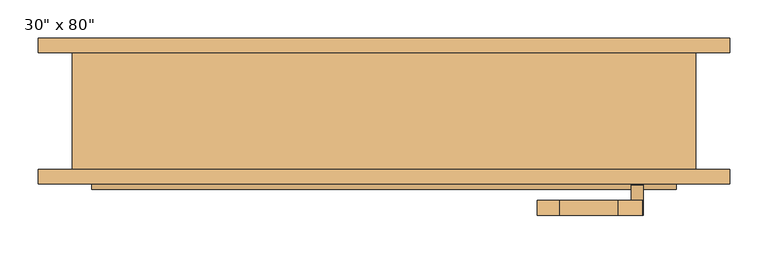
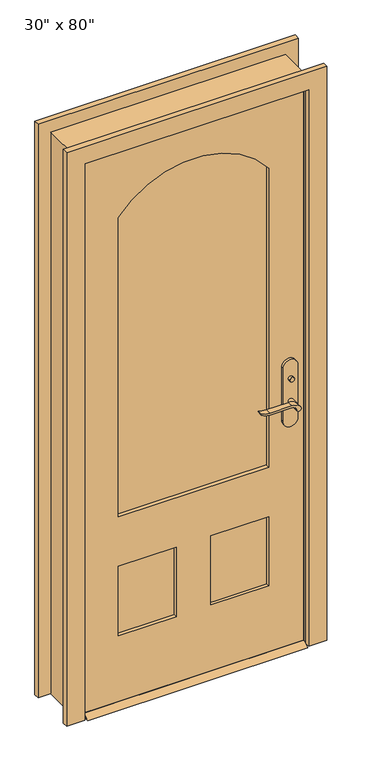
"""IFC4 building model written with IfcOpenShell, lengths in millimetres: door geometry."""

from ifc_helpers import new_model, si_unit, point, frame, frame_2d, origin, place, context, project, spatial, polyline, circle_curve, trimmed, segment, composite_curve, outline, extrude, faceted_brep, source, transform, mapped, element, save


def door_4b146b56(model_context):
    return source(origin(), model_context, "Body", "SolidModel", [
        extrude(outline(polyline([(-38.1, 12.7), (-12.7, 0.0), (-98.425, 0.0), (-73.025, 12.7), (-38.1, 12.7)])), frame((-381.0, 0.0, 0.0), z_axis=(1.0, 0.0, 0.0), x_axis=(0.0, 1.0, 0.0)), (0.0, 0.0, 1.0), 762.0),
        extrude(outline(polyline([(335.2, -18.1), (335.2, -28.1), (325.2, -28.1), (325.2, -18.1), (335.2, -18.1)])), frame((0.0, 0.0, 981.9), z_axis=(0.0, 0.0, 1.0), x_axis=(1.0, 0.0, 0.0)), (0.0, 0.0, 1.0), 30.0),
        extrude(outline(composite_curve([segment(trimmed(circle_curve(frame_2d((996.9, 330.2)), 8.0), [point((996.9, 322.2))], [point((996.9, 338.2))], False, "CARTESIAN"), True, "CONTINUOUS"), segment(trimmed(circle_curve(frame_2d((996.9, 330.2)), 8.0), [point((996.9, 338.2))], [point((996.9, 322.2))], False, "CARTESIAN"), True, "CONTINUOUS")], self_intersect=False)), frame((0.0, -93.025, 0.0), z_axis=(0.0, 1.0, 0.0), x_axis=(0.0, 0.0, 1.0)), (0.0, 0.0, 1.0), 10.0),
        extrude(outline(composite_curve([segment(trimmed(circle_curve(frame_2d((897.1555521, 306.5324871)), 37.2832219), [point((919.0523287, 336.7081363))], [point((934.4, 304.8325667))], False, "CARTESIAN"), True, "CONTINUOUS"), segment(polyline([(934.4, 304.8325667), (934.4, 228.5564091)]), True, "CONTINUOUS"), segment(trimmed(circle_curve(frame_2d((1017.6850638, 228.6227909)), 83.2850902), [point((934.4, 228.5564091))], [point((939.4, 200.2))], True, "CARTESIAN"), True, "CONTINUOUS"), segment(polyline([(939.4, 200.2), (936.6135558, 200.2)]), True, "CONTINUOUS"), segment(trimmed(circle_curve(frame_2d((986.6709207, 232.1396612)), 59.3791355), [point((936.6135558, 200.2))], [point((927.4, 228.5564091))], False, "CARTESIAN"), True, "CONTINUOUS"), segment(polyline([(927.4, 228.5564091), (927.4, 304.8138099)]), True, "CONTINUOUS"), segment(trimmed(circle_curve(frame_2d((909.2738613, 304.8138099)), 18.1261387), [point((927.4, 304.8138099))], [point((914.4, 322.2))], True, "CARTESIAN"), True, "CONTINUOUS"), segment(trimmed(circle_curve(frame_2d((914.4, 330.2)), 8.0), [point((914.4, 322.2))], [point((919.0523287, 336.7081363))], False, "CARTESIAN"), True, "CONTINUOUS")], self_intersect=False)), frame((0.0, 1.9, 0.0), z_axis=(0.0, 1.0, 0.0), x_axis=(0.0, 0.0, 1.0)), (0.0, 0.0, 1.0), 20.0),
        extrude(outline(composite_curve([segment(trimmed(circle_curve(frame_2d((914.4, 330.2)), 8.0), [point((914.3999903, 322.2))], [point((919.0523287, 336.7081363))], False, "CARTESIAN"), True, "CONTINUOUS"), segment(trimmed(circle_curve(frame_2d((897.1555521, 306.5324871)), 37.2832219), [point((919.0523287, 336.7081363))], [point((934.4, 304.8325667))], False, "CARTESIAN"), True, "CONTINUOUS"), segment(polyline([(934.4, 304.8325667), (934.4, 228.5564091)]), True, "CONTINUOUS"), segment(trimmed(circle_curve(frame_2d((1017.6850638, 228.6227909)), 83.2850902), [point((934.4, 228.5564091))], [point((939.4, 200.2))], True, "CARTESIAN"), True, "CONTINUOUS"), segment(polyline([(939.4, 200.2), (936.6135558, 200.2)]), True, "CONTINUOUS"), segment(trimmed(circle_curve(frame_2d((986.6709207, 232.1396612)), 59.3791355), [point((936.6135558, 200.2))], [point((927.4, 228.5564091))], False, "CARTESIAN"), True, "CONTINUOUS"), segment(polyline([(927.4, 228.5564091), (927.4, 304.8138122)]), True, "CONTINUOUS"), segment(trimmed(circle_curve(frame_2d((909.2738682, 304.8138122)), 18.1261318), [point((927.4, 304.8138122))], [point((914.3999903, 322.2))], True, "CARTESIAN"), True, "CONTINUOUS")], self_intersect=False)), frame((0.0, -133.025, 0.0), z_axis=(0.0, 1.0, 0.0), x_axis=(0.0, 0.0, 1.0)), (0.0, 0.0, 1.0), 20.0),
        extrude(outline(composite_curve([segment(trimmed(circle_curve(frame_2d((914.4, 330.2)), 8.0), [point((914.4, 322.2))], [point((914.4, 338.2))], False, "CARTESIAN"), True, "CONTINUOUS"), segment(trimmed(circle_curve(frame_2d((914.4, 330.2)), 8.0), [point((914.4, 338.2))], [point((914.4, 322.2))], False, "CARTESIAN"), True, "CONTINUOUS")], self_intersect=False)), frame((0.0, -28.1, 0.0), z_axis=(0.0, 1.0, 0.0), x_axis=(0.0, 0.0, 1.0)), (0.0, 0.0, 1.0), 30.0),
        extrude(outline(composite_curve([segment(trimmed(circle_curve(frame_2d((914.4, 330.2)), 8.0), [point((914.4, 322.2))], [point((914.4, 338.2))], False, "CARTESIAN"), True, "CONTINUOUS"), segment(trimmed(circle_curve(frame_2d((914.4, 330.2)), 8.0), [point((914.4, 338.2))], [point((914.4, 322.2))], False, "CARTESIAN"), True, "CONTINUOUS")], self_intersect=False)), frame((0.0, -113.025, 0.0), z_axis=(0.0, 1.0, 0.0), x_axis=(0.0, 0.0, 1.0)), (0.0, 0.0, 1.0), 30.0),
        extrude(outline(composite_curve([segment(polyline([(844.4, 355.2), (1039.4, 355.2)]), True, "CONTINUOUS"), segment(trimmed(circle_curve(frame_2d((1039.4, 330.2)), 25.0), [point((1039.4, 355.2))], [point((1039.4, 305.2))], False, "CARTESIAN"), True, "CONTINUOUS"), segment(polyline([(1039.4, 305.2), (844.4, 305.2)]), True, "CONTINUOUS"), segment(trimmed(circle_curve(frame_2d((844.4, 330.2)), 25.0), [point((844.4, 305.2))], [point((844.4, 355.2))], False, "CARTESIAN"), True, "CONTINUOUS")], self_intersect=False)), frame((0.0, -38.1, 0.0), z_axis=(0.0, 1.0, 0.0), x_axis=(0.0, 0.0, 1.0)), (0.0, 0.0, 1.0), 10.0),
        extrude(outline(composite_curve([segment(polyline([(844.4, 355.2), (1039.4, 355.2)]), True, "CONTINUOUS"), segment(trimmed(circle_curve(frame_2d((1039.4, 330.2)), 25.0), [point((1039.4, 355.2))], [point((1039.4, 305.2))], False, "CARTESIAN"), True, "CONTINUOUS"), segment(polyline([(1039.4, 305.2), (844.4, 305.2)]), True, "CONTINUOUS"), segment(trimmed(circle_curve(frame_2d((844.4, 330.2)), 25.0), [point((844.4, 305.2))], [point((844.4, 355.2))], False, "CARTESIAN"), True, "CONTINUOUS")], self_intersect=False)), frame((0.0, -83.025, 0.0), z_axis=(0.0, 1.0, 0.0), x_axis=(0.0, 0.0, 1.0)), (0.0, 0.0, 1.0), 10.0),
        extrude(outline(polyline([(2032.0, -381.0), (12.7, -381.0), (12.7, 381.0), (2032.0, 381.0), (2032.0, -381.0)]), holes=[composite_curve([segment(polyline([(688.975, -260.35), (1784.35, -260.35)]), True, "CONTINUOUS"), segment(trimmed(circle_curve(frame_2d((1580.99125, 0.0)), 330.35875), [point((1784.35, -260.35))], [point((1784.35, 260.35))], True, "CARTESIAN"), True, "CONTINUOUS"), segment(polyline([(1784.35, 260.35), (688.975, 260.35), (688.975, -260.35)]), True, "CONTINUOUS")], self_intersect=False), polyline([(508.0, -60.325), (254.0, -60.325), (254.0, -260.35), (508.0, -260.35), (508.0, -60.325)]), polyline([(508.0, 260.35), (254.0, 260.35), (254.0, 60.325), (508.0, 60.325), (508.0, 260.35)])]), frame((0.0, -73.025, 0.0), z_axis=(0.0, 1.0, 0.0), x_axis=(0.0, 0.0, 1.0)), (0.0, 0.0, 1.0), 34.925),
        faceted_brep([(406.4, -73.025, 0.0), (381.0, -73.025, 0.0), (381.0, -38.1, 0.0), (368.3, -38.1, 0.0), (368.3, -3.175, 0.0), (381.0, -3.175, 0.0), (381.0, 79.375, 0.0), (406.4, 79.375, 0.0), (406.4, 79.375, 2057.4), (406.4, -73.025, 2057.4), (381.0, 79.375, 2032.0), (-381.0, 79.375, 2032.0), (-381.0, 79.375, 0.0), (-406.4, 79.375, 0.0), (-406.4, 79.375, 2057.4), (381.0, -3.175, 2032.0), (368.3, -3.175, 2019.3), (-368.3, -3.175, 2019.3), (-368.3, -3.175, 0.0), (-381.0, -3.175, 0.0), (-381.0, -3.175, 2032.0), (368.3, -38.1, 2019.3), (381.0, -38.1, 2032.0), (-381.0, -38.1, 2032.0), (-381.0, -38.1, 0.0), (-368.3, -38.1, 0.0), (-368.3, -38.1, 2019.3), (381.0, -73.025, 2032.0), (-406.4, -73.025, 2057.4), (-406.4, -73.025, 0.0), (-381.0, -73.025, 0.0), (-381.0, -73.025, 2032.0)], [[[0, 1, 2, 3, 4, 5, 6, 7]], [[7, 8, 9, 0]], [[6, 10, 11, 12, 13, 14, 8, 7]], [[5, 15, 10, 6]], [[4, 16, 17, 18, 19, 20, 15, 5]], [[3, 21, 16, 4]], [[2, 22, 23, 24, 25, 26, 21, 3]], [[1, 27, 22, 2]], [[0, 9, 28, 29, 30, 31, 27, 1]], [[8, 14, 28, 9]], [[15, 20, 11, 10]], [[21, 26, 17, 16]], [[27, 31, 23, 22]], [[29, 13, 12, 19, 18, 25, 24, 30]], [[14, 13, 29, 28]], [[20, 19, 12, 11]], [[26, 25, 18, 17]], [[31, 30, 24, 23]]]),
        extrude(outline(polyline([(-60.325, -49.7416667), (-60.325, -61.3833333), (-260.35, -61.3833333), (-260.35, -49.7416667), (-60.325, -49.7416667)])), frame((0.0, 0.0, 254.0), z_axis=(0.0, 0.0, 1.0), x_axis=(1.0, 0.0, 0.0)), (0.0, 0.0, 1.0), 254.0),
        extrude(outline(polyline([(260.35, -49.7416667), (260.35, -61.3833333), (60.325, -61.3833333), (60.325, -49.7416667), (260.35, -49.7416667)])), frame((0.0, 0.0, 254.0), z_axis=(0.0, 0.0, 1.0), x_axis=(1.0, 0.0, 0.0)), (0.0, 0.0, 1.0), 254.0),
        extrude(outline(composite_curve([segment(polyline([(688.975, -260.35), (688.975, 260.35), (1784.35, 260.35)]), True, "CONTINUOUS"), segment(trimmed(circle_curve(frame_2d((1580.99125, 0.0)), 330.35875), [point((1784.35, 260.35))], [point((1784.35, -260.35))], False, "CARTESIAN"), True, "CONTINUOUS"), segment(polyline([(1784.35, -260.35), (688.975, -260.35)]), True, "CONTINUOUS")], self_intersect=False)), frame((0.0, -59.055, 0.0), z_axis=(0.0, 1.0, 0.0), x_axis=(0.0, 0.0, 1.0)), (0.0, 0.0, 1.0), 6.985),
        extrude(outline(polyline([(0.0, -387.35), (2038.35, -387.35), (2038.35, 387.35), (0.0, 387.35), (0.0, 450.85), (2101.85, 450.85), (2101.85, -450.85), (0.0, -450.85), (0.0, -387.35)])), frame((0.0, 79.375, 0.0), z_axis=(0.0, 1.0, 0.0), x_axis=(0.0, 0.0, 1.0)), (0.0, 0.0, 1.0), 19.05),
        extrude(outline(polyline([(0.0, -387.35), (2038.35, -387.35), (2038.35, 387.35), (0.0, 387.35), (0.0, 450.85), (2101.85, 450.85), (2101.85, -450.85), (0.0, -450.85), (0.0, -387.35)])), frame((0.0, -92.075, 0.0), z_axis=(0.0, 1.0, 0.0), x_axis=(0.0, 0.0, 1.0)), (0.0, 0.0, 1.0), 19.05),
    ])


if __name__ == "__main__":
    model = new_model("IFC4")
    model_context = context("Model", 3, world=origin())
    ifc_project = project(units=[si_unit("LENGTHUNIT", "METRE", prefix="MILLI")], contexts=[model_context])
    site = spatial("IfcSite", under=ifc_project)
    building = spatial("IfcBuilding", under=site)
    placement = place(None, origin())
    door_shape = door_4b146b56(model_context)
    element("IfcDoor", 1, ObjectType="30\" x 80\"", at=placement, inside=building, context=model_context, shape_type="MappedRepresentation", body=[
        mapped(door_shape, transform((0.0, 0.0, 0.0), x_axis=(1.0, 0.0, 0.0), y_axis=(0.0, 1.0, 0.0), z_axis=(0.0, 0.0, 1.0))),
    ])
    save(model, "model.ifc")

# Revit data of these elements
# Type "30\" x 80\""
#   Type Mark = "9"
#   Assembly Code = "B2030100"
#   Analytic Construction = "French door, wood frame with single glass"
#   Threshold Offset [instance default] = 0' - 0 1/2"
#   Thickness = 0' - 1 3/8"
#   Thermal Resistance (R) = 1.0696 (h·ft²·°F)/BTU
#   Swing Angle [instance default] = 90.00°
#   Stiles = 0' - 4 3/4"
#   Rough Width = 2' - 8"
#   Rough Height = 6' - 9"
#   Radius = 1' - 1.00625"
#   Lock Rail = 0' - 7 1/8"
#   Height = 6' - 8"
#   Width = 2' - 6"
#   Heat Transfer Coefficient (U) = 0.9350 BTU/(h·ft²·°F)
#   Door Offset [instance default] = 0' - 0"
#   Bottom Rail = 0' - 9 1/2"
#   Threshold [instance default] = yes
#   Function = 1
#   Exterior Trim [instance default] = yes
#   Trim Material = Cherry
#   Threshold Material = Cherry
#   Panel Material = Cherry
#   Glazing = Glass
#   Frame Material = Cherry
#   Door Handle Material = Aluminum
#   Visual Light Transmittance = 0
#   Solar Heat Gain Coefficient = 0
#   Wall Closure = (empty or 0)
#   Construction Type = (empty or 0)
# Element 1 (IfcDoor, "30\" x 80\"")
#   Materials on its faces: "Cherry", "Aluminum", "Glass"
# Materials
#   "Cherry": class "Wood", colour RGB 226 177 128, transparency 0, Description = "Prunus Serotina", Cost = 0
#   "Glass": class "Glass", colour RGB 0 128 192, transparency 0.75, Description = "Soda Lime Glass", Cost = 0
#   "Aluminum": class "Metal", colour RGB 247 247 247, transparency 0, Description = "Aluminum 6061", Cost = 0
